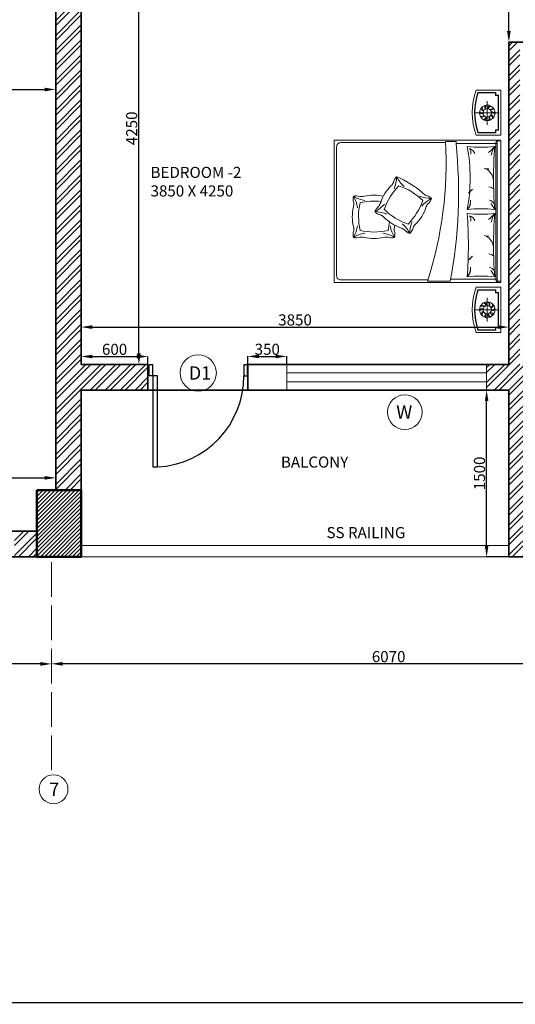
# Model space of a CAD drawing. Units: millimetres. Extents: x -3326 to 29338, y -16792 to 6002.
# Tile 13 of 21: x 16958 to 21421, y -16792 to -7931. Entities that reach past the tile are written whole.
import ezdxf

# ---------------------------------------------------------------- set-up
doc = ezdxf.new("R2010")
doc.units = ezdxf.units.MM
doc.header["$PDMODE"] = 35
doc.header["$PDSIZE"] = 5
doc.linetypes.add('ACAD_ISO04W100', pattern=[30, 24, -3, 0, -3])
for name, color, linetype, lineweight in [('A-ANNO-DIMS', 2, 'Continuous', 13), ('A-ANNO-SYMB', 7, 'Continuous', 18), ('A-AREA-IDEN', 7, 'Continuous', 18), ('A-COLS', 1, 'Continuous', 50), ('A-COLS-PATT', 251, 'Continuous', 13), ('A-DOOR', 3, 'Continuous', 25), ('A-FLOR-RAIL', 8, 'Continuous', 20), ('A-GLAZ', 4, 'Continuous', 18), ('A-GRID', 8, 'ACAD_ISO04W100', 13), ('A-GRID-IDEN', 7, 'Continuous', 18), ('A-WALL', 7, 'Continuous', 35), ('A-WALL-PATT', 252, 'Continuous', 13), ('furn', 28, 'Continuous', 18), ('txt', 7, 'Continuous', 18)]:
    doc.layers.add(name, color=color, linetype=linetype, lineweight=lineweight)
doc.styles.get("Standard").update_dxf_attribs({"font": 'arial.ttf'})
doc.dimstyles.new('ISO-25', dxfattribs={"dimtxt": 100, "dimasz": 100, "dimexe": 1.25, "dimexo": 0.625, "dimtad": 1, "dimtxsty": 'Standard', "dimcen": 2.5, "dimadec": 0, "dimazin": 0, "dimtfac": 1, "dimtmove": 0, "dimatfit": 3, "dimfxl": 1, "dimarcsym": 0})
pattern_1 = [(45, (-10476.65, 1e-12), (-67.35192, 67.35192), []), (45, (-10431.74, 1e-12), (-67.35192, 67.35192), [])]

# ---------------------------------------------------------------- blocks, each defined once
blk = doc.blocks.new('A$C0CE462CD')
for p, q in [((860, 100), (860, 0)), ((860, 0), (893.9, 0))]:
    blk.add_line(p, q)
for points in [[(860, 100), (860, 920), (818.4, 920), (818.4, 100)], [(0, 10), (6.1, 10), (6.1, 90), (0, 90)], [(893.9, 10), (900, 10), (900, 90), (893.9, 90)]]:
    blk.add_lwpolyline(points, close=True)
for points in [[(6.1, 0), (40, 0), (40, 100), (6.1, 100)], [(6.1, 100), (6.1, 0)], [(860, 100), (893.9, 100), (893.9, 0)]]:
    blk.add_lwpolyline(points)
blk.add_arc((859.1, 101.9), 819.1, 92.8508, 180.13091)
blk = doc.blocks.new('*D26')
at = {"layer": 'A-ANNO-DIMS', "color": 0, "lineweight": -2, "transparency": 16777216}
for p, q in [((21361.7, -11264), (21161.1, -11264)), ((21162.3, -12664), (21162.3, -11364)), ((21361.7, -12764), (21161.1, -12764))]:
    blk.add_line(p, q, dxfattribs=at)
at = {"layer": 'A-ANNO-DIMS', "color": 0, "transparency": 16777216}
for points in [[(21145.6, -11364), (21179, -11364), (21162.3, -11264)], [(21145.6, -12664), (21179, -12664), (21162.3, -12764)]]:
    blk.add_solid(points, dxfattribs=at)
at = {"layer": 'Defpoints', "color": 0, "transparency": 16777216}
for p in [(21162.3, -11264), (21362.3, -11264), (21362.3, -12764)]:
    blk.add_point(p, dxfattribs=at)
at = {"layer": 'A-ANNO-DIMS', "color": 0, "transparency": 16777216, "insert": (21110.6, -12014), "char_height": 100, "attachment_point": 5, "rotation": 90}
blk.add_mtext('1500', dxfattribs=at)
blk = doc.blocks.new('*D27')
at = {"layer": 'A-ANNO-DIMS', "color": 0, "lineweight": -2, "transparency": 16777216}
for p, q in [((19012.3, -11033.3), (19012.3, -10960.4)), ((19112.3, -10961.6), (19262.3, -10961.6)), ((19362.3, -11033.3), (19362.3, -10960.4))]:
    blk.add_line(p, q, dxfattribs=at)
at = {"layer": 'A-ANNO-DIMS', "color": 0, "transparency": 16777216}
for points in [[(19112.3, -10944.9), (19112.3, -10978.3), (19012.3, -10961.6)], [(19262.3, -10944.9), (19262.3, -10978.3), (19362.3, -10961.6)]]:
    blk.add_solid(points, dxfattribs=at)
at = {"layer": 'Defpoints', "color": 0, "transparency": 16777216}
for p in [(19362.3, -10961.6), (19012.3, -11034), (19362.3, -11034)]:
    blk.add_point(p, dxfattribs=at)
at = {"layer": 'A-ANNO-DIMS', "color": 0, "transparency": 16777216, "insert": (19187.3, -10909.9), "char_height": 100, "attachment_point": 5}
blk.add_mtext('350', dxfattribs=at)
blk = doc.blocks.new('*D28')
at = {"layer": 'A-ANNO-DIMS', "color": 0, "lineweight": -2, "transparency": 16777216}
for p, q in [((17512.3, -11033.3), (17512.3, -10961)), ((17612.3, -10962.2), (18012.3, -10962.2)), ((18112.3, -11033.3), (18112.3, -10961))]:
    blk.add_line(p, q, dxfattribs=at)
at = {"layer": 'A-ANNO-DIMS', "color": 0, "transparency": 16777216}
for points in [[(17612.3, -10945.6), (17612.3, -10978.9), (17512.3, -10962.2)], [(18012.3, -10945.6), (18012.3, -10978.9), (18112.3, -10962.2)]]:
    blk.add_solid(points, dxfattribs=at)
at = {"layer": 'Defpoints', "color": 0, "transparency": 16777216}
for p in [(18112.3, -10962.2), (17512.3, -11034), (18112.3, -11034)]:
    blk.add_point(p, dxfattribs=at)
at = {"layer": 'A-ANNO-DIMS', "color": 0, "transparency": 16777216, "insert": (17812.3, -10910.6), "char_height": 100, "attachment_point": 5}
blk.add_mtext('600', dxfattribs=at)
blk = doc.blocks.new('*D30')
at = {"layer": 'A-ANNO-DIMS', "color": 0, "lineweight": -2, "transparency": 16777216}
for p, q in [((21362.9, -6784), (21363.6, -6784)), ((21362.3, -8034), (21362.3, -6884)), ((21362.9, -8134), (21363.6, -8134))]:
    blk.add_line(p, q, dxfattribs=at)
at = {"layer": 'A-ANNO-DIMS', "color": 0, "transparency": 16777216}
for points in [[(21345.6, -6884), (21379, -6884), (21362.3, -6784)], [(21345.6, -8034), (21379, -8034), (21362.3, -8134)]]:
    blk.add_solid(points, dxfattribs=at)
at = {"layer": 'Defpoints', "color": 0, "transparency": 16777216}
for p in [(21362.3, -6784), (21362.3, -6784), (21362.3, -8134)]:
    blk.add_point(p, dxfattribs=at)
at = {"layer": 'A-ANNO-DIMS', "color": 0, "transparency": 16777216, "insert": (21310.6, -7459), "char_height": 100, "attachment_point": 5, "rotation": 90}
blk.add_mtext('1350', dxfattribs=at)
blk = doc.blocks.new('*D34')
at = {"layer": 'A-ANNO-DIMS', "color": 0, "lineweight": -2, "transparency": 16777216}
for p, q in [((17512.3, -10608.6), (17512.3, -10698.8)), ((17612.3, -10697.5), (21262.3, -10697.5)), ((21362.3, -10715.1), (21362.3, -10696.3))]:
    blk.add_line(p, q, dxfattribs=at)
at = {"layer": 'A-ANNO-DIMS', "color": 0, "transparency": 16777216}
for points in [[(17612.3, -10680.8), (17612.3, -10714.2), (17512.3, -10697.5)], [(21262.3, -10680.8), (21262.3, -10714.2), (21362.3, -10697.5)]]:
    blk.add_solid(points, dxfattribs=at)
at = {"layer": 'Defpoints', "color": 0, "transparency": 16777216}
for p in [(17512.3, -10608), (21362.3, -10697.5), (21362.3, -10715.8)]:
    blk.add_point(p, dxfattribs=at)
at = {"layer": 'A-ANNO-DIMS', "color": 0, "transparency": 16777216, "insert": (19437.3, -10645.8), "char_height": 100, "attachment_point": 5}
blk.add_mtext('3850', dxfattribs=at)
blk = doc.blocks.new('*D35')
at = {"layer": 'A-ANNO-DIMS', "color": 0, "lineweight": -2, "transparency": 16777216}
for p, q in [((17512.9, -6784), (18032.6, -6784)), ((18031.3, -10934), (18031.3, -6884)), ((17512.9, -11034), (18032.6, -11034))]:
    blk.add_line(p, q, dxfattribs=at)
at = {"layer": 'A-ANNO-DIMS', "color": 0, "transparency": 16777216}
for points in [[(18014.6, -6884), (18048, -6884), (18031.3, -6784)], [(18014.6, -10934), (18048, -10934), (18031.3, -11034)]]:
    blk.add_solid(points, dxfattribs=at)
at = {"layer": 'Defpoints', "color": 0, "transparency": 16777216}
for p in [(17512.3, -6784), (18031.3, -6784), (17512.3, -11034)]:
    blk.add_point(p, dxfattribs=at)
at = {"layer": 'A-ANNO-DIMS', "color": 0, "transparency": 16777216, "insert": (17979.6, -8909), "char_height": 100, "attachment_point": 5, "rotation": 90}
blk.add_mtext('4250', dxfattribs=at)
blk = doc.blocks.new('*D38')
at = {"layer": 'A-ANNO-DIMS', "color": 0, "lineweight": -2, "transparency": 16777216}
for p, q in [((15536.7, -12053.5), (15536.7, -12052.9)), ((15636.7, -12054.2), (17182.3, -12054.2)), ((17282.3, -12053.5), (17282.3, -12052.9))]:
    blk.add_line(p, q, dxfattribs=at)
at = {"layer": 'A-ANNO-DIMS', "color": 0, "transparency": 16777216}
for points in [[(15636.7, -12037.5), (15636.7, -12070.8), (15536.7, -12054.2)], [(17182.3, -12037.5), (17182.3, -12070.8), (17282.3, -12054.2)]]:
    blk.add_solid(points, dxfattribs=at)
at = {"layer": 'Defpoints', "color": 0, "transparency": 16777216}
for p in [(15536.7, -12054.2), (17282.3, -12054.2), (17282.3, -12054.2)]:
    blk.add_point(p, dxfattribs=at)
at = {"layer": 'A-ANNO-DIMS', "color": 0, "transparency": 16777216, "insert": (16409.5, -11993.4), "char_height": 100, "attachment_point": 5}
blk.add_mtext('1745,58', dxfattribs=at)
blk = doc.blocks.new('*D48')
at = {"layer": 'A-ANNO-DIMS', "color": 0, "lineweight": -2, "transparency": 16777216}
for p, q in [((13962.3, -8558.9), (13962.3, -8558.2)), ((14062.3, -8559.5), (17182.3, -8559.5)), ((17282.3, -8558.9), (17282.3, -8558.2))]:
    blk.add_line(p, q, dxfattribs=at)
at = {"layer": 'A-ANNO-DIMS', "color": 0, "transparency": 16777216}
for points in [[(14062.3, -8542.8), (14062.3, -8576.1), (13962.3, -8559.5)], [(17182.3, -8542.8), (17182.3, -8576.1), (17282.3, -8559.5)]]:
    blk.add_solid(points, dxfattribs=at)
at = {"layer": 'Defpoints', "color": 0, "transparency": 16777216}
for p in [(13962.3, -8559.5), (17282.3, -8559.5), (17282.3, -8559.5)]:
    blk.add_point(p, dxfattribs=at)
at = {"layer": 'A-ANNO-DIMS', "color": 0, "transparency": 16777216, "insert": (15622.3, -8507.8), "char_height": 100, "attachment_point": 5}
blk.add_mtext('3320', dxfattribs=at)
blk = doc.blocks.new('*D158')
at = {"layer": 'A-ANNO-DIMS', "color": 0, "lineweight": -2, "transparency": 16777216}
for p, q in [((17245, -13726.9), (17245, -13726.3)), ((23215, -13727.6), (17345, -13727.6)), ((23315, -13726.9), (23315, -13726.3))]:
    blk.add_line(p, q, dxfattribs=at)
at = {"layer": 'A-ANNO-DIMS', "color": 0, "transparency": 16777216}
for points in [[(17345, -13710.9), (17345, -13744.2), (17245, -13727.6)], [(23215, -13710.9), (23215, -13744.2), (23315, -13727.6)]]:
    blk.add_solid(points, dxfattribs=at)
at = {"layer": 'Defpoints', "color": 0, "transparency": 16777216}
for p in [(17245, -13727.6), (17245, -13727.6), (23315, -13727.6)]:
    blk.add_point(p, dxfattribs=at)
at = {"layer": 'A-ANNO-DIMS', "color": 0, "transparency": 16777216, "insert": (20280, -13675.9), "char_height": 100, "attachment_point": 5}
blk.add_mtext('6070', dxfattribs=at)
blk = doc.blocks.new('*D159')
at = {"layer": 'A-ANNO-DIMS', "color": 0, "lineweight": -2, "transparency": 16777216}
for p, q in [((11527.3, -13721), (11527.3, -13729.7)), ((17145, -13728.4), (11627.3, -13728.4)), ((17245, -13721), (17245, -13729.7))]:
    blk.add_line(p, q, dxfattribs=at)
at = {"layer": 'A-ANNO-DIMS', "color": 0, "transparency": 16777216}
for points in [[(11627.3, -13711.8), (11627.3, -13745.1), (11527.3, -13728.4)], [(17145, -13711.8), (17145, -13745.1), (17245, -13728.4)]]:
    blk.add_solid(points, dxfattribs=at)
at = {"layer": 'Defpoints', "color": 0, "transparency": 16777216}
for p in [(11527.3, -13720.4), (11527.3, -13728.4), (17245, -13720.4)]:
    blk.add_point(p, dxfattribs=at)
at = {"layer": 'A-ANNO-DIMS', "color": 0, "transparency": 16777216, "insert": (14386.1, -13667.7), "char_height": 100, "attachment_point": 5}
blk.add_mtext('5717,66', dxfattribs=at)
blk = doc.blocks.new('BED-WITH-NIGHTSTANDS')
for p, q in [((1378.9, 2083.2), (1378.9, 1869.8)), ((1272.3, 1976.5), (1485.6, 1976.5)), ((1466.8, 1702.3), (1097.4, 1702.3)), ((1455.8, 1708.6), (1455.8, 473.4)), ((1466.8, 480.5), (1049.3, 480.5)), ((1378.9, 98.8), (1378.9, 312.2)), ((1272.2, 205.5), (1485.6, 205.5))]:
    blk.add_line(p, q)
for points in [[(1279.5, 2182), (1501.4, 2182), (1501.4, 1775.2), (1279.5, 1775.2, -0.181818)], [(1097.4, 1719.6), (1097.4, 1702.3, -0.072944), (1045.8, 463.1), (840.6, 463.1, 0.092568), (1003.3, 1719.6)], [(1198.4, 1674.1, 0.058596), (1445.6, 1674.1, 0.036889), (1445.6, 1107.7, 0.052163), (1198.4, 1107.7, 0.093111)], [(1198.4, 1070.9, 0.058596), (1445.6, 1070.9, 0.036648), (1445.6, 500.8, 0.052163), (1198.4, 500.8, 0.036967)], [(1279.6, 0), (1501.5, 0), (1501.5, 406.8), (1279.6, 406.8, 0.181818)]]:
    blk.add_lwpolyline(points, format="xyb", close=True)
for points in [[(1454.8, 1797.4), (1295, 1797.4, -0.167087), (1295, 2159.8), (1454.8, 2159.8)], [(1454.8, 1799.6), (1296.6, 1799.6, -0.165559), (1296.6, 2157.6), (1454.8, 2157.6)], [(1003.9, 1708.6), (59.2, 1708.6, 0.414214), (22.2, 1671.6), (22.2, 510.4, 0.414214), (59.2, 473.4), (844.2, 473.4)], [(540, 1293.1, 0.091296), (562.8, 1401.4, 0.091296), (630.7, 1314.1, 0.091296)], [(583.2, 1320, 0.111006), (451.8, 1108.7, 0.119549), (665.6, 975.5, 0.107813), (797.5, 1186.1)], [(797.2, 1187.3, 0.121865), (583.2, 1319.9, 0.121865)], [(211.2, 1122.2, 0.091296), (173.3, 1226.2, 0.091296), (277.2, 1187.9, 0.091296)], [(233.7, 1167.8, 0.111006), (234, 919, 0.119549), (485.8, 919, 0.033212), (497.4, 995.5)], [(475.6, 1065.1, 0.091296), (367.2, 1087.5, 0.091296), (454.4, 1155.8)], [(768.3, 1228.3, 0.091296), (876.7, 1205.8, 0.091296), (789.5, 1137.6, 0.091296)], [(367.2, 1087.5, 0.159461), (418, 1058.9, -0.076283), (449.6, 1036.2, 0.115075), (598.7, 943.3, -0.076283), (633, 924.9, 0.159461), (681.1, 892)], [(703.9, 1000.2, 0.091296), (681.1, 892, 0.091296), (613.2, 979.3, 0.091296)], [(277.2, 894.6, 0.091296), (173.3, 856.3, 0.091296), (211.2, 960.3)], [(505.3, 960.3, 0.091296), (543.2, 856.3, 0.091296), (439.3, 894.6, 0.091296)], [(173.3, 856.3, 0.159461), (231.6, 858.9, -0.076283), (270.5, 856.3, 0.115075), (446, 856.3, -0.076283), (484.9, 858.9, 0.159461), (543.2, 856.3)], [(1454.9, 384.6), (1295.1, 384.6, 0.167087), (1295.1, 22.2), (1454.9, 22.2)], [(1454.9, 382.4), (1296.7, 382.4, 0.165559), (1296.7, 24.4), (1454.9, 24.4)]]:
    blk.add_lwpolyline(points, format="xyb")
for points in [[(1479.2, 2133.2), (1452.6, 2133.2), (1452.6, 2159.8)], [(1479.2, 2135.4), (1454.8, 2135.4), (1454.8, 2159.8)], [(1477, 2135.4), (1477, 1821.8)], [(1479.2, 2135.4), (1479.2, 1821.8)], [(1479.2, 1824), (1452.6, 1824), (1452.6, 1797.4)], [(1479.2, 1821.8), (1454.8, 1821.8), (1454.8, 1797.4)], [(1501.5, 1730.8), (0, 1730.8), (0, 451.2), (1501.5, 451.2)], [(1501.5, 463.1), (1466.8, 463.1), (1466.8, 1723.4), (1501.5, 1723.4), (1501.5, 451.2)], [(1479.3, 358), (1452.7, 358), (1452.7, 384.6)], [(1479.3, 360.2), (1454.9, 360.2), (1454.9, 384.6)], [(1477.1, 46.6), (1477.1, 360.2)], [(1479.3, 46.6), (1479.3, 360.2)], [(1479.3, 48.8), (1452.7, 48.8), (1452.7, 22.2)], [(1479.3, 46.6), (1454.9, 46.6), (1454.9, 22.2)]]:
    blk.add_lwpolyline(points)
for centre, radius in [((1378.9, 1976.5), 69.7), ((1378.9, 1976.5), 37.8), ((1378.9, 205.5), 69.7), ((1378.9, 205.5), 37.8)]:
    blk.add_circle(centre, radius)
for centre, radius, start, end in [((1400.9, 2024.2), 44.8, 154.17003, 200.48975), ((1396.5, 2024.6), 34.1, 142.30017, 202.53802), ((1424.8, 2002.2), 44.8, 118.17003, 164.48975), ((1421.4, 2005.1), 34.1, 106.30017, 166.53802), ((1340.3, 2012.2), 44.8, 226.17003, 272.48975), ((1338.5, 2008.1), 34.1, 214.30017, 274.53802), ((1327.7, 1978.3), 34.1, 250.30017, 310.53802), ((1368.7, 2028), 44.8, 190.17003, 236.48975), ((1364.8, 2025.8), 34.1, 178.30017, 238.53802), ((1431.1, 1970.3), 44.8, 82.17003, 128.48975), ((1430.1, 1974.7), 34.1, 70.30017, 130.53802), ((1393, 1927.2), 34.1, 358.30017, 58.53802), ((1389.2, 1925), 44.8, 10.17003, 56.48975), ((1417.5, 1940.8), 44.8, 46.17003, 92.48975), ((1419.3, 1944.9), 34.1, 34.30017, 94.53802), ((1326.7, 1982.7), 44.8, 262.17003, 308.48975), ((1336.4, 1947.9), 34.1, 286.30017, 346.53802), ((1333.1, 1950.8), 44.8, 298.17003, 344.48975), ((1361.4, 1928.3), 34.1, 322.30017, 22.53802), ((1356.9, 1928.8), 44.8, 334.17003, 20.48975), ((1478, 1708.6), 22.2, 90, 180), ((1175.6, 1619.4), 56.2, 346.48229, 38.55627), ((1192.7, 1576.7), 82.2, 24.2916, 70.9896), ((1214.5, 1859.4), 296.3, 306.49353, 321.27919), ((1652.3, 1542.6), 244.9, 147.53791, 167.5233), ((1375.3, 1532.7), 61.4, 245.89274, 286.11919), ((1299.1, 1354.7), 137.1, 6.68493, 58.3182), ((419.7, 1408.4), 128.4, 315.77185, 333.2208), ((626.3, 1332.5), 93.8, 132.65224, 168.89294), ((256.3, 651.7), 810, 48.38179, 67.76439), ((785.6, 1046.2), 386.5, 135.13065, 161.38844), ((884.1, 1348.9), 128.4, 225.58539, 243.03435), ((1208.9, 1279), 20.7, 263.75428, 347.21866), ((1026.5, 1507.4), 308.8, 306.20852, 315.08491), ((1377, 1216.1), 96.2, 51.81741, 79.89867), ((263.7, 1201.2), 93.8, 164.57915, 200.81985), ((198.5, 1135.9), 93.8, 69.36661, 105.60731), ((48.2, 1156.4), 128.4, 347.69876, 5.14771), ((242.7, 1351.6), 128.4, 265.03874, 282.4877), ((360.8, 659.2), 524.3, 83.19556, 104.02838), ((358.2, 849.8), 386.5, 76.87111, 103.12889), ((298.1, 1211.9), 128.4, 323.29829, 340.74724), ((807.5, 1142.5), 93.8, 42.46578, 78.70648), ((947.4, 1081.9), 128.4, 143.29829, 160.74724), ((789.7, 1230.6), 90.5, 307.29372, 344.09733), ((1127.7, 1179.9), 101.1, 314.40604, 6.83423), ((1163, 1161), 64, 303.63488, 0.84559), ((1363.4, 1094.5), 103.5, 40.53543, 70.35581), ((1276.2, 1030), 186.4, 24.64565, 44.15848), ((550.3, 1042.5), 386.5, 167.05756, 193.31535), ((468.2, 1051.5), 107.3, 128.77541, 160.35713), ((460, 1247.6), 386.5, 315.13065, 341.38844), ((1214.5, 1256.2), 296.3, 306.49353, 321.27919), ((1652.3, 939.4), 244.9, 147.53791, 167.5233), ((825.9, 885.4), 128.4, 135.77185, 153.2208), ((1175.6, 1016.2), 56.2, 346.48229, 38.55627), ((1192.7, 973.5), 82.2, 24.2916, 70.9896), ((278.1, 879.2), 107.3, 160.70232, 192.28404), ((48.9, 925.3), 128.4, 355.2252, 12.67415), ((669.5, 927.3), 128.4, 167.69876, 185.14771), ((461.1, 884), 86.6, 341.39955, 21.57741), ((167.4, 1041.2), 386.5, 347.05756, 348.7033), ((626.1, 958.8), 86.6, 309.47264, 349.6505), ((1375.3, 929.5), 61.4, 245.89274, 286.11919), ((1299.1, 751.6), 137.1, 6.68493, 58.3182), ((1208.9, 675.8), 20.7, 263.75428, 347.21866), ((1026.5, 904.2), 308.8, 306.20852, 315.08491), ((1377, 612.9), 96.2, 51.81741, 79.89867), ((1127.7, 576.7), 101.1, 314.40604, 6.83423), ((1163, 557.8), 64, 303.63488, 0.84559), ((1363.4, 491.3), 103.5, 40.53543, 70.35581), ((1276.2, 426.8), 186.4, 24.64565, 44.15848), ((1478, 473.4), 22.2, 180, 270), ((1336.4, 234.2), 34.1, 13.46198, 73.69983), ((1333, 231.2), 44.8, 15.51025, 61.82997), ((1361.4, 253.7), 34.1, 337.46198, 37.69983), ((1356.9, 253.2), 44.8, 339.51025, 25.82997), ((1340.3, 169.8), 44.8, 87.51025, 133.82997), ((1338.5, 173.9), 34.1, 85.46198, 145.69983), ((1327.7, 203.7), 34.1, 49.46198, 109.69983), ((1326.7, 199.3), 44.8, 51.51025, 97.82997), ((1368.6, 154), 44.8, 123.51025, 169.82997), ((1364.8, 156.2), 34.1, 121.46198, 181.69983), ((1430.1, 207.3), 34.1, 229.46198, 289.69983), ((1393, 254.8), 34.1, 301.46198, 1.69983), ((1389.2, 257.1), 44.8, 303.51025, 349.82997), ((1417.5, 241.2), 44.8, 267.51025, 313.82997), ((1419.3, 237.1), 34.1, 265.46198, 325.69983), ((1402.8, 152.7), 44.8, 159.51025, 205.82997), ((1398.4, 152.3), 34.1, 157.46198, 217.69983), ((1426.7, 174.7), 44.8, 195.51025, 241.82997), ((1423.3, 171.8), 34.1, 193.46198, 253.69983), ((1433, 206.6), 44.8, 231.51025, 277.82997)]:
    blk.add_arc(centre, radius, start, end)
blk = doc.blocks.new('TAG-D1')
blk.add_circle((163.3, 163.3), 163.3)
at = {"insert": (78, 223.5), "char_height": 120, "attachment_point": 1}
blk.add_mtext_dynamic_manual_height_columns('D1', width=137.943, gutter_width=12.5, heights=[0], dxfattribs=at)
blk = doc.blocks.new('TAG-W')
blk.add_circle((156.8, 156.8), 156.8)
at = {"insert": (79.7, 216.8), "char_height": 120, "attachment_point": 1}
blk.add_mtext_dynamic_manual_height_columns('W', width=376.575, gutter_width=12.5, heights=[0], dxfattribs=at)
blk = doc.blocks.new('GLAZ-1800x80')
for p, q in [((0, 80), (1800, 80)), ((0, 0), (1800, 0))]:
    blk.add_line(p, q)
blk = doc.blocks.new('*D235')
at = {"layer": 'A-ANNO-DIMS', "color": 0, "lineweight": -2, "transparency": 16777216}
for p, q in [((-617.7, -12764.6), (-617.7, -16776.1)), ((29282.3, -12764.6), (29282.3, -16776.1)), ((-517.7, -16774.9), (29182.3, -16774.9))]:
    blk.add_line(p, q, dxfattribs=at)
at = {"layer": 'A-ANNO-DIMS', "color": 0, "transparency": 16777216}
for points in [[(-517.7, -16758.2), (-517.7, -16791.6), (-617.7, -16774.9)], [(29182.3, -16758.2), (29182.3, -16791.6), (29282.3, -16774.9)]]:
    blk.add_solid(points, dxfattribs=at)
at = {"layer": 'Defpoints', "color": 0, "transparency": 16777216}
for p in [(-617.7, -12764), (29282.3, -12764), (29282.3, -16774.9)]:
    blk.add_point(p, dxfattribs=at)
at = {"layer": 'A-ANNO-DIMS', "color": 0, "transparency": 16777216, "insert": (14332.3, -16723.2), "char_height": 100, "attachment_point": 5}
blk.add_mtext('29900', dxfattribs=at)

msp = doc.modelspace()

# ---------------------------------------------------------------- hatches: boundary and pattern name
at = {"layer": 'A-COLS-PATT'}
h = msp.add_hatch(dxfattribs=at)
h.set_pattern_fill('ANSI31', color=256, scale=8)
h.set_pattern_definition([(45, (-24609, -5556.948), (-17.960512, 17.960512), [])])
h.paths.add_polyline_path([(17112.301, -12763.952), (17512.301, -12763.952), (17512.301, -12163.952), (17112.301, -12163.952)])
at = {"layer": 'A-WALL-PATT'}
h = msp.add_hatch(dxfattribs=at)
h.set_pattern_fill('ANSI32', color=256, scale=10)
h.set_pattern_definition(pattern_1)
h.paths.add_polyline_path([(12212.301, -1983.952), (11640.861, -1983.952), (11640.861, -2213.952), (12212.301, -2213.952)])
h.paths.add_polyline_path([(14712.301, -1983.952), (14012.301, -1983.952), (14012.301, -2213.952), (14712.301, -2213.952)])
h.paths.add_polyline_path([(17012.301, -1983.952), (16512.301, -1983.952), (16512.301, -2213.952), (17012.301, -2213.952)])
h.paths.add_polyline_path([(11382.301, -2383.952), (11040.861, -2383.952), (7302.301, -2383.952), (7302.301, -1935.766), (7217.026, -1935.766), (7202.301, -1933.952), (7202.301, -2483.952), (7302.301, -2483.952), (11152.301, -2483.952), (11152.301, -2833.952), (11283.549, -2833.952), (11283.549, -2830.395), (11363.875, -2830.395), (11382.301, -2833.952)])
h.paths.add_polyline_path([(11382.301, -3733.952), (11363.875, -3733.952), (11363.875, -3734.058), (11283.549, -3734.058), (11152.301, -3733.952), (11152.301, -6450.401), (11382.301, -6450.401)])
h.paths.add_polyline_path([(13462.301, -6450.401), (12606.738, -6450.401), (11382.301, -6450.401), (11382.301, -6680.401), (12606.738, -6680.401), (13462.301, -6680.401)])
h.paths.add_polyline_path([(11382.301, -7050.401), (11152.301, -7050.401), (11152.301, -8810.401), (11382.301, -8810.401)])
h.paths.add_polyline_path([(13462.301, -8980.401), (11751.174, -8980.401), (11751.174, -9210.401), (13462.301, -9210.401)])
h.paths.add_polyline_path([(13962.301, -6850.401), (13732.301, -6850.401), (13732.301, -7350.401), (13962.301, -7350.401)])
h.paths.add_polyline_path([(13962.301, -8309.482), (13732.301, -8309.482), (13732.301, -8809.482), (13962.301, -8809.482)])
h.paths.add_polyline_path([(15712.301, -12533.952), (12902.301, -12533.952), (12902.301, -12763.952), (15712.301, -12763.952)])
h.paths.add_polyline_path([(11508.301, -9211.585), (11382.301, -9211.585), (11152.301, -9211.585), (11152.301, -11033.952), (10952.301, -11033.952), (10952.301, -11263.952), (11152.301, -11263.952), (11152.301, -12361.585), (11508.301, -12361.585)])
h.paths.add_polyline_path([(12002.301, -12533.952), (11902.301, -12533.952), (11902.301, -12761.585), (11152.301, -12761.585), (11152.301, -12763.952), (11902.301, -12763.952), (12002.301, -12763.952)])
h.paths.add_polyline_path([(17112.301, -12533.952), (16912.301, -12533.952), (16912.301, -12763.952), (17112.301, -12763.952)])
h.paths.add_polyline_path([(11382.301, 3596.048), (11152.301, 3596.048), (11152.301, 2096.048), (11382.301, 2096.048)])
h.paths.add_polyline_path([(11382.301, 1496.048), (11152.301, 1496.048), (11152.301, -1983.952), (11382.301, -1983.952)])
h = msp.add_hatch(dxfattribs=at)
h.set_pattern_fill('ANSI32', color=256, scale=10)
h.set_pattern_definition(pattern_1)
h.paths.add_polyline_path([(29282.301, -7283.952), (28882.301, -7283.952), (28882.301, -7383.952), (29052.301, -7383.952), (29052.301, -10763.952), (29282.301, -10763.952)])
h.paths.add_polyline_path([(29282.301, -11263.952), (29052.301, -11263.952), (29052.301, -12763.952), (29282.301, -12763.952)])
h.paths.add_polyline_path([(25052.301, -11263.952), (25652.301, -11263.952), (25652.301, -11123.904), (25652.289, -11123.904), (25652.289, -11033.952), (25052.301, -11033.952), (24572.301, -11033.952), (24572.301, -11263.952), (24822.301, -11263.952), (24822.301, -12763.952), (25052.301, -12763.952)])
h.paths.add_polyline_path([(26902.301, -11033.952), (26552.301, -11033.952), (26552.301, -11263.952), (26902.301, -11263.952)])
h.paths.add_polyline_path([(21992.301, -6683.952), (21362.301, -6683.952), (17512.301, -6683.952), (17512.301, -6783.952), (21362.301, -6783.952), (21992.301, -6783.952)])
h.paths.add_polyline_path([(17512.301, -7283.952), (17282.301, -7283.952), (17282.301, -12163.952), (17512.301, -12163.952), (17512.301, -11263.952), (18112.301, -11263.952), (18112.301, -11033.952), (17512.301, -11033.952)])
h.paths.add_polyline_path([(21462.301, -8211.864), (21462.064, -8211.864), (21462.064, -8142.609), (21462.301, -8133.952), (21362.301, -8133.952), (21362.301, -8233.952), (21362.301, -11033.952), (21162.301, -11033.952), (21162.301, -11263.952), (21362.301, -11263.952), (21362.301, -12763.952), (21592.301, -12763.952), (21592.301, -11263.952), (21992.301, -11263.952), (21992.301, -11033.952), (21592.301, -11033.952), (21462.301, -11033.952)])
h.paths.add_polyline_path([(24152.301, -8133.952), (23322.301, -8133.952), (23322.301, -7433.952), (23092.301, -7433.952), (23092.301, -8133.952), (22241.021, -8133.952), (22241.021, -8142.609), (22241.182, -8142.609), (22241.182, -8211.864), (22241.021, -8233.952), (23092.301, -8233.952), (23092.301, -10513.206), (23322.301, -10513.206), (23322.301, -8233.952), (24152.301, -8233.952)])
h.paths.add_polyline_path([(25052.301, -8233.952), (25052.301, -8133.952), (24952.301, -8133.952), (24952.301, -11033.952), (25052.301, -11033.952)])
h.paths.add_polyline_path([(23972.301, -11033.952), (23493.251, -11033.952), (23493.251, -11263.952), (23972.301, -11263.952)])
h.paths.add_polyline_path([(23092.301, -11033.952), (22592.301, -11033.952), (22592.301, -11263.952), (23092.301, -11263.952)])
h.paths.add_polyline_path([(28882.301, -11033.952), (28702.301, -11033.952), (28702.301, -11263.952), (28882.301, -11263.952)])
h.paths.add_polyline_path([(17512.301, -3883.952), (17387.589, -3883.952), (17387.589, -3888.07), (17282.301, -3888.07), (17282.301, -6683.952), (17512.301, -6683.952)])
h.paths.add_polyline_path([(21462.301, -2183.952), (21362.301, -2183.952), (21362.301, -2383.952), (17282.301, -2383.952), (17282.301, -2483.952), (17512.301, -2483.952), (21462.301, -2483.952)])
h.paths.add_polyline_path([(17512.301, -2483.952), (17282.301, -2483.952), (17282.301, -2833.952), (17512.301, -2833.952)])
h.paths.add_polyline_path([(21462.301, 1866.048), (21992.301, 1866.048), (21992.301, 2096.048), (21592.301, 2096.048), (21592.301, 3596.048), (21362.301, 3596.048), (21362.301, 1866.048), (21362.301, -1283.952), (21462.301, -1283.952)])
h.paths.add_polyline_path([(17512.301, 1496.048), (17282.301, 1496.048), (17282.301, -1983.952), (17612.301, -1983.952), (17612.301, -1883.952), (17512.301, -1883.952)])
h.paths.add_polyline_path([(17512.301, 3596.048), (17282.301, 3596.048), (17282.301, 2096.048), (17512.301, 2096.048)])
h.paths.add_polyline_path([(18135.023, 2096.048), (17685.023, 2096.048), (17685.023, 1866.048), (18135.023, 1866.048), (18135.023, 1876.048), (18128.942, 1876.048), (18128.942, 1956.048), (18135.023, 1956.048)])
h.paths.add_polyline_path([(19385.023, 2096.048), (19035.023, 2096.048), (19035.023, 1866.048), (19385.023, 1866.048)])
h.paths.add_polyline_path([(21362.301, 2096.048), (21185.023, 2096.048), (21185.023, 1866.048), (21362.301, 1866.048)])
h.paths.add_polyline_path([(23092.301, 2096.048), (22592.301, 2096.048), (22592.301, 1866.048), (23092.301, 1866.048)])
h.paths.add_polyline_path([(23972.301, 2096.048), (23492.301, 2096.048), (23492.301, 1866.048), (23972.301, 1866.048)])
h.paths.add_polyline_path([(23972.301, 2496.048), (23872.301, 2496.048), (23872.301, 2096.048), (23972.301, 2096.048)])
h.paths.add_polyline_path([(22692.301, 2496.048), (22592.301, 2496.048), (22592.301, 2096.048), (22692.301, 2096.048)])
h.paths.add_polyline_path([(23322.301, 1346.048), (23092.301, 1346.048), (23092.301, -1733.952), (23322.301, -1733.952)])
h.paths.add_polyline_path([(23092.301, -933.952), (22262.301, -933.952), (22262.301, -1033.952), (23092.301, -1033.952)])
h.paths.add_polyline_path([(24952.301, -1433.952), (24952.301, -1733.952), (23492.301, -1733.952), (23492.301, -1833.952), (24952.301, -1833.952), (24952.301, -2483.952), (25052.301, -2483.952), (25052.301, -2466.23), (25049.26, -2466.23), (25049.26, -2386.23), (25049.941, -1433.952)])
h.paths.add_polyline_path([(22692.301, -11263.952), (22592.301, -11263.952), (22592.301, -11663.952), (22692.301, -11663.952)])
h.paths.add_polyline_path([(23972.301, -11263.952), (23872.301, -11263.952), (23872.301, -11663.952), (23972.301, -11663.952)])

# ---------------------------------------------------------------- linework, layer by layer
at = {"layer": 'A-COLS'}
msp.add_lwpolyline([(17112.301, -12163.952), (17512.301, -12163.952), (17512.301, -12763.952), (17112.301, -12763.952)], close=True, dxfattribs=at)
at = {"layer": 'A-FLOR-RAIL'}
for p, q in [((21362.301, -12663.952), (17512.301, -12663.952)), ((21362.301, -12763.952), (17512.301, -12763.952))]:
    msp.add_line(p, q, dxfattribs=at)
at = {"layer": 'A-GLAZ'}
for p, q in [((19362.301, -11033.952), (19362.301, -11263.952)), ((21162.301, -11033.952), (21162.301, -11263.952))]:
    msp.add_line(p, q, dxfattribs=at)
at = {"layer": 'A-GRID', "ltscale": 13}
msp.add_line((17244.966, -14684.889), (17244.966, -12755.956), dxfattribs=at)
at = {"layer": 'A-GRID-IDEN'}
msp.add_circle((17262.792, -14856.272), 130.151, dxfattribs=at)
at = {"layer": 'A-WALL'}
for p, q in [((17512.301, -3883.952), (17512.301, -11033.952)), ((17282.301, -7283.952), (17282.301, -12163.952)), ((23092.301, -8133.952), (21362.301, -8133.952)), ((21362.301, -8133.952), (21362.301, -8233.952)), ((21362.301, -8233.952), (21362.301, -11033.952)), ((18112.301, -11033.952), (17512.301, -11033.952)), ((18112.301, -11033.952), (18112.301, -11263.952)), ((21362.301, -11033.952), (19012.301, -11033.952)), ((19012.301, -11033.952), (19012.301, -11263.952)), ((21362.301, -11263.952), (17512.301, -11263.952)), ((17512.301, -11263.952), (17512.301, -12763.952)), ((21362.301, -11263.952), (21362.301, -12763.952)), ((17112.301, -12533.952), (11902.301, -12533.952)), ((17112.301, -12763.952), (11902.301, -12763.952)), ((17512.301, -12763.952), (17112.301, -12763.952)), ((21592.301, -12763.952), (21362.301, -12763.952))]:
    msp.add_line(p, q, dxfattribs=at)

# ---------------------------------------------------------------- block references
at = {"layer": 'A-ANNO-SYMB'}
for name, p in [('TAG-D1', (18401.949, -11273.5)), ('TAG-W', (20268.701, -11619.541))]:
    msp.add_blockref(name, p, dxfattribs=at)
at = {"layer": 'A-DOOR', "rotation": 180}
msp.add_blockref('A$C0CE462CD', (19016.354, -11035.792), dxfattribs=at)
at = {"layer": 'A-GLAZ'}
msp.add_blockref('GLAZ-1800x80', (19362.301, -11188.952), dxfattribs=at)
at = {"layer": 'furn'}
msp.add_blockref('BED-WITH-NIGHTSTANDS', (19789.125, -10746.327), dxfattribs=at)

# ---------------------------------------------------------------- texts
at = {"layer": 'A-AREA-IDEN', "char_height": 100, "attachment_point": 1}
for s, insert in [('BEDROOM -2\\P3850 X 4250', (18136.429, -9255.437)), ('BALCONY', (19310.382, -11862.223))]:
    msp.add_mtext_dynamic_manual_height_columns(s, width=1168.90663, gutter_width=12.5, heights=[0], dxfattribs=dict(at, insert=insert))
at = {"layer": 'A-GRID-IDEN', "insert": (17223.952, -14796.272), "char_height": 120, "attachment_point": 1}
msp.add_mtext_dynamic_manual_height_columns('7', width=551.68587, gutter_width=12.5, heights=[0], dxfattribs=at)
at = {"layer": 'txt', "insert": (19720.799, -12496.982), "char_height": 100, "attachment_point": 1}
msp.add_mtext_dynamic_manual_height_columns('SS RAILING', width=1168.90663, gutter_width=12.5, heights=[0], dxfattribs=at)

# ---------------------------------------------------------------- dimensions: what is measured, and where the dimension line sits
at = {"layer": 'A-ANNO-DIMS'}
for base, p1, p2, picture, middle in [((18031.303, -6783.952), (17512.301, -11033.952), (17512.301, -6783.952), '*D35', (17979.62, -8908.952)), ((21362.301, -6783.952), (21362.301, -8133.952), (21362.301, -6783.952), '*D30', (21310.584, -7458.952)), ((21162.301, -11263.952), (21362.301, -12763.952), (21362.301, -11263.952), '*D26', (21110.618, -12013.952))]:
    dim = msp.add_linear_dim(base=base, p1=p1, p2=p2, angle=90, dimstyle='ISO-25', override={"dimclrd": 0, "dimclre": 0, "dimclrt": 0}, dxfattribs=at)
    dim.commit()
    dim.dimension.update_dxf_attribs({"geometry": picture, "text_midpoint": middle})
for base, p1, p2, override, picture, middle in [((17282.301, -8559.482), (13962.301, -8559.482), (17282.301, -8559.482), {"dimclrd": 0, "dimclre": 0, "dimclrt": 0}, '*D48', (15622.301, -8507.765)), ((21362.301, -10697.509), (17512.301, -10607.979), (21362.301, -10715.772), {"dimclrd": 0, "dimclre": 0, "dimclrt": 0}, '*D34', (19437.301, -10645.792)), ((18112.301, -10962.238), (17512.301, -11033.952), (18112.301, -11033.952), {"dimclrd": 0, "dimclre": 0, "dimclrt": 0}, '*D28', (17812.301, -10910.556)), ((19362.301, -10961.613), (19012.301, -11033.952), (19362.301, -11033.952), {"dimclrd": 0, "dimclre": 0, "dimclrt": 0}, '*D27', (19187.301, -10909.896)), ((17282.301, -12054.152), (15536.718, -12054.152), (17282.301, -12054.152), {"dimclrd": 0, "dimclre": 0, "dimclrt": 0}, '*D38', (16409.509, -11993.432)), ((29282.301, -16774.892), (-617.699, -12763.952), (29282.301, -12763.952), {"dimdec": 0, "dimlfac": 1, "dimrnd": 0, "dimzin": 0, "dimdsep": 46, "dimlunit": 2}, '*D235', (14332.301, -16723.21)), ((11527.3007, -13728.4186), (17244.9656, -13720.4224), (11527.3007, -13720.4224), {"dimclrd": 0, "dimclre": 0, "dimclrt": 0}, '*D159', (14386.1331, -13667.6981)), ((17244.966, -13727.562), (23314.966, -13727.562), (17244.966, -13727.562), {"dimclrd": 0, "dimclre": 0, "dimclrt": 0}, '*D158', (20279.966, -13675.88))]:
    dim = msp.add_linear_dim(base=base, p1=p1, p2=p2, dimstyle='ISO-25', override=override, dxfattribs=at)
    dim.commit()
    dim.dimension.update_dxf_attribs({"geometry": picture, "text_midpoint": middle})

doc.saveas('drawing.dxf')
